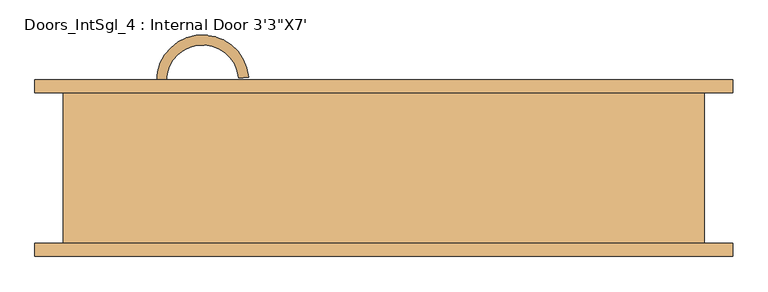
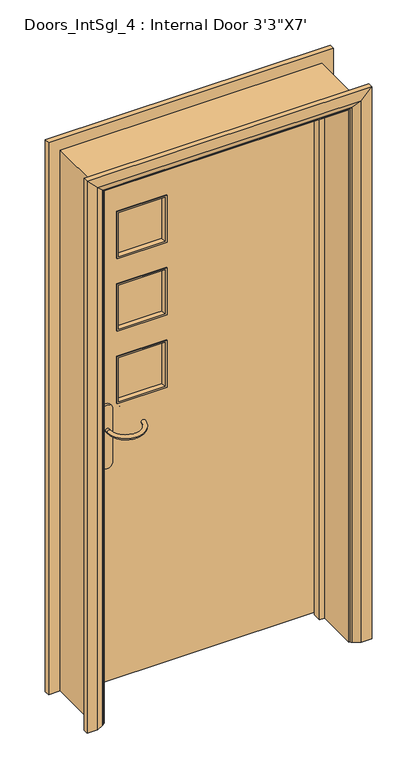
"""IFC4 building model written with IfcOpenShell, lengths in millimetres: door geometry."""

from ifc_helpers import new_model, si_unit, point, frame, frame_2d, origin, place, context, project, spatial, polyline, circle_curve, ellipse_curve, trimmed, segment, composite_curve, outline, extrude, faceted_brep, source, transform, mapped, element, save
from ifc_brep_helpers import plane_surface, cylinder_surface, revolved_surface, advanced_brep


def door_3dbecc4b(model_context):
    return source(origin(), model_context, "Body", "SolidModel", [
        advanced_brep(
        [(-345.5, 68.3, 1000.0), (-330.5, 68.3, 1000.0), (-330.5, 58.3, 1000.0), (-345.5, 58.3, 1000.0), (-205.5986682, 52.1917759, 1000.0), (-220.5415886, 53.4991121, 1000.0)],
        [
            (0, 1, circle_curve(frame((-338.0, 68.3, 1000.0), z_axis=(0.0, 1.0, 0.0), x_axis=(1.0, 0.0, 0.0)), 7.5)),
            (1, 0, circle_curve(frame((-338.0, 68.3, 1000.0), z_axis=(0.0, 1.0, 0.0), x_axis=(1.0, 0.0, 0.0)), 7.5)),
            (1, 2),
            (2, 3, circle_curve(frame((-338.0, 58.3, 1000.0), z_axis=(0.0, 1.0, 0.0), x_axis=(1.0, 0.0, 0.0)), 7.5)),
            (3, 0),
            (3, 2, circle_curve(frame((-338.0, 58.3, 1000.0), z_axis=(0.0, 1.0, 0.0), x_axis=(1.0, 0.0, 0.0)), 7.5)),
            (4, 5, circle_curve(frame((-213.0701284, 52.845444, 1000.0), z_axis=(0.08715574274766678, 0.9961946980917448, 0.0), x_axis=(-0.9961946980917448, 0.08715574274766678, 0.0)), 7.5)),
            (5, 4, circle_curve(frame((-213.0701284, 52.845444, 1000.0), z_axis=(0.08715574274766678, 0.9961946980917448, 0.0), x_axis=(-0.9961946980917448, 0.08715574274766678, 0.0)), 7.5)),
            (4, 3, circle_curve(frame((-275.4159887, 58.3, 1000.0), z_axis=(0.0, 0.0, -1.0), x_axis=(-1.0, 0.0, 0.0)), 70.0840113)),
            (2, 5, circle_curve(frame((-275.4159887, 58.3, 1000.0), z_axis=(0.0, 0.0, 1.0), x_axis=(-1.0, 0.0, 0.0)), 55.0840113)),
        ],
        [
            plane_surface(frame((-338.0, 68.3, 1000.0), z_axis=(0.0, 1.0, 0.0), x_axis=(0.0, 0.0, 1.0))),
            cylinder_surface(frame((-338.0, 68.3, 1000.0), z_axis=(0.0, 1.0, 0.0), x_axis=(1.0, 0.0, 0.0)), 7.5),
            plane_surface(frame((-213.0701284, 52.845444, 1000.0), z_axis=(0.08715574274766678, 0.9961946980917448, 0.0), x_axis=(0.0, 0.0, 1.0))),
            revolved_surface(trimmed(ellipse_curve(frame((-338.0, 58.3, 1000.0), z_axis=(0.0, -1.0, 0.0), x_axis=(1.0, 0.0, 0.0)), 7.5, 7.5), [point((-345.5, 58.3, 1000.0))], [point((-330.5, 58.3, 1000.0))], True, "CARTESIAN"), (-275.4159887, 58.3, 1000.0), (0.0, 0.0, -1.0)),
            revolved_surface(trimmed(ellipse_curve(frame((-338.0, 58.3, 1000.0), z_axis=(0.0, -1.0, 0.0), x_axis=(1.0, 0.0, 0.0)), 7.5, 7.5), [point((-330.5, 58.3, 1000.0))], [point((-345.5, 58.3, 1000.0))], True, "CARTESIAN"), (-275.4159887, 58.3, 1000.0), (0.0, 0.0, -1.0)),
        ],
        [
            (0, [[1, 2]]),
            (1, [[3, 4, 5, -2]]),
            (1, [[-5, 6, -3, -1]]),
            (2, [[7, 8]]),
            (3, [[-7, 9, -4, 10]]),
            (4, [[-8, -10, -6, -9]]),
        ],
    ),
        extrude(outline(composite_curve([segment(trimmed(circle_curve(frame_2d((870.0, -338.0)), 20.0), [point((870.0, -358.0))], [point((870.0, -318.0))], False, "CARTESIAN"), True, "CONTINUOUS"), segment(polyline([(870.0, -318.0), (1080.0, -318.0)]), True, "CONTINUOUS"), segment(trimmed(circle_curve(frame_2d((1080.0, -338.0)), 20.0), [point((1080.0, -318.0))], [point((1080.0, -358.0))], False, "CARTESIAN"), True, "CONTINUOUS"), segment(polyline([(1080.0, -358.0), (870.0, -358.0)]), True, "CONTINUOUS")], self_intersect=False)), frame((0.0, 68.3, 0.0), z_axis=(0.0, 1.0, 0.0), x_axis=(0.0, 0.0, 1.0)), (0.0, 0.0, 1.0), 8.0),
        advanced_brep(
        [(-345.5, 122.3, 1000.0), (-330.5, 122.3, 1000.0), (-345.5, 132.3, 1000.0), (-330.5, 132.3, 1000.0), (-205.5986682, 138.4082241, 1000.0), (-220.5415886, 137.1008879, 1000.0)],
        [
            (0, 1, circle_curve(frame((-338.0, 122.3, 1000.0), z_axis=(0.0, -1.0, 0.0), x_axis=(1.0, 0.0, 0.0)), 7.5)),
            (1, 0, circle_curve(frame((-338.0, 122.3, 1000.0), z_axis=(0.0, -1.0, 0.0), x_axis=(1.0, 0.0, 0.0)), 7.5)),
            (0, 2),
            (2, 3, circle_curve(frame((-338.0, 132.3, 1000.0), z_axis=(0.0, -1.0, 0.0), x_axis=(1.0, 0.0, 0.0)), 7.5)),
            (3, 1),
            (3, 2, circle_curve(frame((-338.0, 132.3, 1000.0), z_axis=(0.0, -1.0, 0.0), x_axis=(1.0, 0.0, 0.0)), 7.5)),
            (4, 5, circle_curve(frame((-213.0701284, 137.754556, 1000.0), z_axis=(0.08715574274766356, -0.9961946980917451, 0.0), x_axis=(-0.9961946980917451, -0.08715574274766356, 0.0)), 7.5)),
            (5, 4, circle_curve(frame((-213.0701284, 137.754556, 1000.0), z_axis=(0.08715574274766356, -0.9961946980917451, 0.0), x_axis=(-0.9961946980917451, -0.08715574274766356, 0.0)), 7.5)),
            (5, 3, circle_curve(frame((-275.4159887, 132.3, 1000.0), z_axis=(0.0, 0.0, 1.0), x_axis=(-1.0, 0.0, 0.0)), 55.0840113)),
            (2, 4, circle_curve(frame((-275.4159887, 132.3, 1000.0), z_axis=(0.0, 0.0, -1.0), x_axis=(-1.0, 0.0, 0.0)), 70.0840113)),
        ],
        [
            plane_surface(frame((-338.0, 122.3, 1000.0), z_axis=(0.0, -1.0, 0.0), x_axis=(0.0, 0.0, 1.0))),
            cylinder_surface(frame((-338.0, 122.3, 1000.0), z_axis=(0.0, -1.0, 0.0), x_axis=(1.0, 0.0, 0.0)), 7.5),
            plane_surface(frame((-213.0701284, 137.754556, 1000.0), z_axis=(0.08715574274766356, -0.9961946980917451, 0.0), x_axis=(0.0, 0.0, 1.0))),
            revolved_surface(trimmed(ellipse_curve(frame((-338.0, 132.3, 1000.0), z_axis=(0.0, -1.0, 0.0), x_axis=(1.0, 0.0, 0.0)), 7.5, 7.5), [point((-345.5, 132.3, 1000.0))], [point((-330.5, 132.3, 1000.0))], True, "CARTESIAN"), (-275.4159887, 132.3, 1000.0), (0.0, 0.0, -1.0)),
            revolved_surface(trimmed(ellipse_curve(frame((-338.0, 132.3, 1000.0), z_axis=(0.0, -1.0, 0.0), x_axis=(1.0, 0.0, 0.0)), 7.5, 7.5), [point((-330.5, 132.3, 1000.0))], [point((-345.5, 132.3, 1000.0))], True, "CARTESIAN"), (-275.4159887, 132.3, 1000.0), (0.0, 0.0, -1.0)),
        ],
        [
            (0, [[1, 2]]),
            (1, [[-1, 3, 4, 5]]),
            (1, [[-2, -5, 6, -3]]),
            (2, [[7, 8]]),
            (3, [[9, -4, 10, -8]]),
            (4, [[-10, -6, -9, -7]]),
        ],
    ),
        extrude(outline(composite_curve([segment(trimmed(circle_curve(frame_2d((870.0, -338.0)), 20.0), [point((870.0, -358.0))], [point((870.0, -318.0))], False, "CARTESIAN"), True, "CONTINUOUS"), segment(polyline([(870.0, -318.0), (1080.0, -318.0)]), True, "CONTINUOUS"), segment(trimmed(circle_curve(frame_2d((1080.0, -338.0)), 20.0), [point((1080.0, -318.0))], [point((1080.0, -358.0))], False, "CARTESIAN"), True, "CONTINUOUS"), segment(polyline([(1080.0, -358.0), (870.0, -358.0)]), True, "CONTINUOUS")], self_intersect=False)), frame((0.0, 114.3, 0.0), z_axis=(0.0, 1.0, 0.0), x_axis=(0.0, 0.0, 1.0)), (0.0, 0.0, 1.0), 8.0),
        extrude(outline(polyline([(2091.6, -453.3), (8.0, -453.3), (8.0, 453.3), (2091.6, 453.3), (2091.6, -453.3)]), holes=[polyline([(1841.6, -113.3), (1656.6, -113.3), (1656.6, -298.3), (1841.6, -298.3), (1841.6, -113.3)]), polyline([(1086.6, -298.3), (1271.6, -298.3), (1271.6, -113.3), (1086.6, -113.3), (1086.6, -298.3)]), polyline([(1556.6, -113.3), (1371.6, -113.3), (1371.6, -298.3), (1556.6, -298.3), (1556.6, -113.3)])]), frame((0.0, 76.3, 0.0), z_axis=(0.0, 1.0, 0.0), x_axis=(0.0, 0.0, 1.0)), (0.0, 0.0, 1.0), 38.0),
        faceted_brep([(-455.3, 114.3, 0.0), (-455.3, -114.3, 0.0), (-487.3, -114.3, 0.0), (-487.3, 114.3, 0.0), (-455.3, 114.3, 2093.6), (-455.3, -114.3, 2093.6), (-487.3, -114.3, 2125.6), (-487.3, 114.3, 2125.6), (455.3, 114.3, 0.0), (487.3, 114.3, 0.0), (487.3, -114.3, 0.0), (455.3, -114.3, 0.0), (455.3, 114.3, 2093.6), (487.3, 114.3, 2125.6), (487.3, -114.3, 2125.6), (455.3, -114.3, 2093.6)], [[[0, 1, 2, 3]], [[1, 0, 4, 5]], [[2, 1, 5, 6]], [[3, 2, 6, 7]], [[0, 3, 7, 4]], [[8, 9, 10, 11]], [[12, 13, 9, 8]], [[13, 14, 10, 9]], [[14, 15, 11, 10]], [[15, 12, 8, 11]], [[5, 4, 12, 15]], [[6, 5, 15, 14]], [[7, 6, 14, 13]], [[4, 7, 13, 12]]]),
        advanced_brep(
        [(-530.3, -134.3, 0.0), (-530.3, -114.3, 0.0), (-460.3, -114.3, 0.0), (-464.3, -120.3, 0.0), (-490.3, -134.3, 0.0), (-530.3, -134.3, 2168.6), (-530.3, -114.3, 2168.6), (-460.3, -114.3, 2098.6), (-464.3, -120.3, 2102.6), (-490.3, -134.3, 2128.6), (530.3, -134.3, 0.0), (490.3, -134.3, 0.0), (464.3, -120.3, 0.0), (460.3, -114.3, 0.0), (530.3, -114.3, 0.0), (530.3, -134.3, 2168.6), (490.3, -134.3, 2128.6), (464.3, -120.3, 2102.6), (460.3, -114.3, 2098.6), (530.3, -114.3, 2168.6)],
        [
            (0, 1),
            (1, 2),
            (2, 3, circle_curve(frame((-468.3, -113.3, 0.0), z_axis=(0.0, 0.0, -1.0), x_axis=(-1.0, 0.0, 0.0)), 8.0622577)),
            (3, 4),
            (4, 0),
            (0, 5),
            (5, 6),
            (6, 1),
            (6, 7),
            (7, 2),
            (7, 8, ellipse_curve(frame((-468.3, -113.3, 2106.6), z_axis=(-0.7071067811865475, 0.0, -0.7071067811865475), x_axis=(0.7071067811865474, 0.0, -0.7071067811865476)), 11.4017543, 8.0622577)),
            (8, 3),
            (8, 9),
            (9, 4),
            (9, 5),
            (10, 11),
            (11, 12),
            (12, 13, circle_curve(frame((468.3, -113.3, 0.0), z_axis=(0.0, 0.0, -1.0), x_axis=(1.0, 0.0, 0.0)), 8.0622577)),
            (13, 14),
            (14, 10),
            (15, 16),
            (16, 11),
            (10, 15),
            (16, 17),
            (17, 12),
            (17, 18, ellipse_curve(frame((468.3, -113.3, 2106.6), z_axis=(0.7071067811865475, 0.0, -0.7071067811865475), x_axis=(0.7071067811865474, 0.0, 0.7071067811865476)), 11.4017543, 8.0622577)),
            (18, 13),
            (18, 19),
            (19, 14),
            (19, 15),
            (5, 15),
            (19, 6),
            (18, 7),
            (17, 8),
            (16, 9),
        ],
        [
            plane_surface(frame((-460.3, -187.1010989, 0.0), z_axis=(0.0, 0.0, -1.0), x_axis=(1.0, 0.0, 0.0))),
            plane_surface(frame((-530.3, -134.3, 0.0), z_axis=(-1.0, 0.0, 0.0), x_axis=(0.0, 0.0, 1.0))),
            plane_surface(frame((-530.3, -114.3, 0.0), z_axis=(0.0, 1.0, 0.0), x_axis=(0.0, 0.0, 1.0))),
            cylinder_surface(frame((-468.3, -113.3, 0.0), z_axis=(0.0, 0.0, -1.0), x_axis=(-1.0, 0.0, 0.0)), 8.0622577),
            plane_surface(frame((-464.3, -120.3, 0.0), z_axis=(0.4740998230350183, -0.8804710999221749, 0.0), x_axis=(0.0, 0.0, 1.0))),
            plane_surface(frame((-490.3, -134.3, 0.0), z_axis=(0.0, -1.0, 0.0), x_axis=(0.0, 0.0, 1.0))),
            plane_surface(frame((460.3, -187.1010989, 0.0), z_axis=(0.0, 0.0, -1.0), x_axis=(-1.0, 0.0, 0.0))),
            plane_surface(frame((490.3, -134.3, 2128.6), z_axis=(0.0, -1.0, 0.0), x_axis=(0.0, 0.0, -1.0))),
            plane_surface(frame((464.3, -120.3, 2102.6), z_axis=(-0.4740998230350183, -0.8804710999221749, 0.0), x_axis=(0.0, 0.0, -1.0))),
            cylinder_surface(frame((468.3, -113.3, 2098.6), z_axis=(0.0, 0.0, 1.0), x_axis=(1.0, 0.0, 0.0)), 8.0622577),
            plane_surface(frame((530.3, -114.3, 2168.6), z_axis=(0.0, 1.0, 0.0), x_axis=(0.0, 0.0, -1.0))),
            plane_surface(frame((530.3, -134.3, 2168.6), z_axis=(1.0, 0.0, 0.0), x_axis=(0.0, 0.0, -1.0))),
            plane_surface(frame((-530.3, -134.3, 2168.6), z_axis=(0.0, 0.0, 1.0), x_axis=(1.0, 0.0, 0.0))),
            plane_surface(frame((-530.3, -114.3, 2168.6), z_axis=(0.0, 1.0, 0.0), x_axis=(1.0, 0.0, 0.0))),
            cylinder_surface(frame((-460.3, -113.3, 2106.6), z_axis=(-1.0, 0.0, 0.0), x_axis=(0.0, 0.0, 1.0)), 8.0622577),
            plane_surface(frame((-464.3, -120.3, 2102.6), z_axis=(0.0, -0.8804710999221749, -0.4740998230350183), x_axis=(1.0, 0.0, 0.0))),
            plane_surface(frame((-490.3, -134.3, 2128.6), z_axis=(0.0, -1.0, 0.0), x_axis=(1.0, 0.0, 0.0))),
        ],
        [
            (0, [[1, 2, 3, 4, 5]]),
            (1, [[-1, 6, 7, 8]]),
            (2, [[-2, -8, 9, 10]]),
            (3, [[-3, -10, 11, 12]]),
            (4, [[-4, -12, 13, 14]]),
            (5, [[-5, -14, 15, -6]]),
            (6, [[16, 17, 18, 19, 20]]),
            (7, [[21, 22, -16, 23]]),
            (8, [[24, 25, -17, -22]]),
            (9, [[26, 27, -18, -25]]),
            (10, [[28, 29, -19, -27]]),
            (11, [[30, -23, -20, -29]]),
            (12, [[-7, 31, -30, 32]]),
            (13, [[-9, -32, -28, 33]]),
            (14, [[-11, -33, -26, 34]]),
            (15, [[-13, -34, -24, 35]]),
            (16, [[-15, -35, -21, -31]]),
        ],
    ),
        extrude(outline(polyline([(0.0, -455.3), (0.0, -436.3), (2074.6, -436.3), (2074.6, 436.3), (0.0, 436.3), (0.0, 455.3), (2093.6, 455.3), (2093.6, -455.3), (0.0, -455.3)])), frame((0.0, 42.3, 0.0), z_axis=(0.0, 1.0, 0.0), x_axis=(0.0, 0.0, 1.0)), (0.0, 0.0, 1.0), 32.0),
        advanced_brep(
        [(530.3, 134.3, 0.0), (530.3, 114.3, 0.0), (460.3, 114.3, 0.0), (464.3, 120.3, 0.0), (490.3, 134.3, 0.0), (530.3, 134.3, 2168.6), (530.3, 114.3, 2168.6), (-530.3, 114.3, 2168.6), (-530.3, 114.3, 0.0), (-460.3, 114.3, 0.0), (-460.3, 114.3, 2098.6), (460.3, 114.3, 2098.6), (464.3, 120.3, 2102.6), (490.3, 134.3, 2128.6), (-490.3, 134.3, 2128.6), (-490.3, 134.3, 0.0), (-530.3, 134.3, 0.0), (-530.3, 134.3, 2168.6), (-464.3, 120.3, 0.0), (-464.3, 120.3, 2102.6)],
        [
            (0, 1),
            (1, 2),
            (2, 3, circle_curve(frame((468.3, 113.3, 0.0), z_axis=(0.0, 0.0, -1.0), x_axis=(1.0, 0.0, 0.0)), 8.0622577)),
            (3, 4),
            (4, 0),
            (0, 5),
            (5, 6),
            (6, 1),
            (6, 7),
            (7, 8),
            (8, 9),
            (9, 10),
            (10, 11),
            (11, 2),
            (11, 12, ellipse_curve(frame((468.3, 113.3, 2106.6), z_axis=(0.7071067811865475, 0.0, -0.7071067811865475), x_axis=(-0.7071067811865474, 0.0, -0.7071067811865476)), 11.4017543, 8.0622577)),
            (12, 3),
            (12, 13),
            (13, 4),
            (13, 14),
            (14, 15),
            (15, 16),
            (16, 17),
            (17, 5),
            (7, 17),
            (16, 8),
            (15, 18),
            (18, 9, circle_curve(frame((-468.3, 113.3, 0.0), z_axis=(0.0, 0.0, -1.0), x_axis=(-1.0, 0.0, 0.0)), 8.0622577)),
            (19, 10, ellipse_curve(frame((-468.3, 113.3, 2106.6), z_axis=(-0.7071067811865475, 0.0, -0.7071067811865475), x_axis=(-0.7071067811865474, 0.0, 0.7071067811865476)), 11.4017543, 8.0622577)),
            (18, 19),
            (14, 19),
            (19, 12),
        ],
        [
            plane_surface(frame((460.3, 114.3, 0.0), z_axis=(0.0, 0.0, -1.0), x_axis=(0.0, -1.0, 0.0))),
            plane_surface(frame((530.3, 134.3, 0.0), z_axis=(1.0, 0.0, 0.0), x_axis=(0.0, 0.0, 1.0))),
            plane_surface(frame((530.3, 114.3, 0.0), z_axis=(0.0, -1.0, 0.0), x_axis=(0.0, 0.0, 1.0))),
            cylinder_surface(frame((468.3, 113.3, 0.0), z_axis=(0.0, 0.0, -1.0), x_axis=(1.0, 0.0, 0.0)), 8.0622577),
            plane_surface(frame((464.3, 120.3, 0.0), z_axis=(-0.4740998230350126, 0.8804710999221779, 0.0), x_axis=(0.0, 0.0, 1.0))),
            plane_surface(frame((490.3, 134.3, 0.0), z_axis=(0.0, 1.0, 0.0), x_axis=(0.0, 0.0, 1.0))),
            plane_surface(frame((-530.3, 134.3, 2168.6), z_axis=(-1.0, 0.0, 0.0), x_axis=(0.0, 0.0, -1.0))),
            plane_surface(frame((-460.3, 114.3, 0.0), z_axis=(0.0, 0.0, -1.0), x_axis=(0.0, -1.0, 0.0))),
            cylinder_surface(frame((-468.3, 113.3, 2098.6), z_axis=(0.0, 0.0, 1.0), x_axis=(-1.0, 0.0, 0.0)), 8.0622577),
            plane_surface(frame((-464.3, 120.3, 2102.6), z_axis=(0.4740998230350183, 0.8804710999221749, 0.0), x_axis=(0.0, 0.0, -1.0))),
            plane_surface(frame((530.3, 134.3, 2168.6), z_axis=(0.0, 0.0, 1.0), x_axis=(-1.0, 0.0, 0.0))),
            cylinder_surface(frame((460.3, 113.3, 2106.6), z_axis=(1.0, 0.0, 0.0), x_axis=(0.0, 0.0, 1.0)), 8.0622577),
            plane_surface(frame((464.3, 120.3, 2102.6), z_axis=(0.0, 0.8804710999221763, -0.4740998230350154), x_axis=(-1.0, 0.0, 0.0))),
        ],
        [
            (0, [[1, 2, 3, 4, 5]]),
            (1, [[-1, 6, 7, 8]]),
            (2, [[-2, -8, 9, 10, 11, 12, 13, 14]]),
            (3, [[-3, -14, 15, 16]]),
            (4, [[-4, -16, 17, 18]]),
            (5, [[-5, -18, 19, 20, 21, 22, 23, -6]]),
            (6, [[24, -22, 25, -10]]),
            (7, [[-21, 26, 27, -11, -25]]),
            (8, [[28, -12, -27, 29]]),
            (9, [[30, -29, -26, -20]]),
            (10, [[-7, -23, -24, -9]]),
            (11, [[-15, -13, -28, 31]]),
            (12, [[-17, -31, -30, -19]]),
        ],
    ),
        faceted_brep([(-113.3, 117.3, 1841.6), (-113.3, 104.3, 1841.6), (-113.3, 104.3, 1656.6), (-113.3, 117.3, 1656.6), (-125.3, 104.3, 1829.6), (-119.3, 117.3, 1835.6), (-119.3, 117.3, 1662.6), (-125.3, 104.3, 1668.6), (-298.3, 104.3, 1656.6), (-298.3, 117.3, 1656.6), (-292.3, 117.3, 1662.6), (-286.3, 104.3, 1668.6), (-298.3, 104.3, 1841.6), (-298.3, 117.3, 1841.6), (-292.3, 117.3, 1835.6), (-286.3, 104.3, 1829.6)], [[[0, 1, 2, 3]], [[4, 5, 6, 7]], [[3, 2, 8, 9]], [[7, 6, 10, 11]], [[9, 8, 12, 13]], [[11, 10, 14, 15]], [[1, 12, 8, 2], [7, 11, 15, 4]], [[13, 12, 1, 0]], [[3, 9, 13, 0], [5, 14, 10, 6]], [[15, 14, 5, 4]]]),
        faceted_brep([(-119.3, 73.3, 1835.6), (-125.3, 86.3, 1829.6), (-125.3, 86.3, 1668.6), (-119.3, 73.3, 1662.6), (-113.3, 86.3, 1841.6), (-113.3, 73.3, 1841.6), (-113.3, 73.3, 1656.6), (-113.3, 86.3, 1656.6), (-286.3, 86.3, 1668.6), (-292.3, 73.3, 1662.6), (-298.3, 73.3, 1656.6), (-298.3, 86.3, 1656.6), (-286.3, 86.3, 1829.6), (-292.3, 73.3, 1835.6), (-298.3, 73.3, 1841.6), (-298.3, 86.3, 1841.6)], [[[0, 1, 2, 3]], [[4, 5, 6, 7]], [[3, 2, 8, 9]], [[7, 6, 10, 11]], [[9, 8, 12, 13]], [[11, 10, 14, 15]], [[13, 12, 1, 0]], [[5, 14, 10, 6], [3, 9, 13, 0]], [[15, 14, 5, 4]], [[7, 11, 15, 4], [1, 12, 8, 2]]]),
        extrude(outline(polyline([(-298.3, 104.3), (-113.3, 104.3), (-113.3, 86.3), (-298.3, 86.3), (-298.3, 104.3)])), frame((0.0, 0.0, 1656.6), z_axis=(0.0, 0.0, 1.0), x_axis=(1.0, 0.0, 0.0)), (0.0, 0.0, 1.0), 185.0),
        extrude(outline(polyline([(-298.3, 104.3), (-113.3, 104.3), (-113.3, 86.3), (-298.3, 86.3), (-298.3, 104.3)])), frame((0.0, 0.0, 1086.6), z_axis=(0.0, 0.0, 1.0), x_axis=(1.0, 0.0, 0.0)), (0.0, 0.0, 1.0), 185.0),
        extrude(outline(polyline([(-298.3, 104.3), (-113.3, 104.3), (-113.3, 86.3), (-298.3, 86.3), (-298.3, 104.3)])), frame((0.0, 0.0, 1371.6), z_axis=(0.0, 0.0, 1.0), x_axis=(1.0, 0.0, 0.0)), (0.0, 0.0, 1.0), 185.0),
        faceted_brep([(-298.3, 117.3, 1371.6), (-298.3, 104.3, 1371.6), (-298.3, 104.3, 1556.6), (-298.3, 117.3, 1556.6), (-286.3, 104.3, 1383.6), (-292.3, 117.3, 1377.6), (-292.3, 117.3, 1550.6), (-286.3, 104.3, 1544.6), (-113.3, 104.3, 1556.6), (-113.3, 117.3, 1556.6), (-119.3, 117.3, 1550.6), (-125.3, 104.3, 1544.6), (-113.3, 104.3, 1371.6), (-113.3, 117.3, 1371.6), (-119.3, 117.3, 1377.6), (-125.3, 104.3, 1383.6)], [[[0, 1, 2, 3]], [[4, 5, 6, 7]], [[3, 2, 8, 9]], [[7, 6, 10, 11]], [[9, 8, 12, 13]], [[11, 10, 14, 15]], [[1, 12, 8, 2], [7, 11, 15, 4]], [[13, 12, 1, 0]], [[3, 9, 13, 0], [5, 14, 10, 6]], [[15, 14, 5, 4]]]),
        faceted_brep([(-298.3, 117.3, 1086.6), (-298.3, 104.3, 1086.6), (-298.3, 104.3, 1271.6), (-298.3, 117.3, 1271.6), (-286.3, 104.3, 1098.6), (-292.3, 117.3, 1092.6), (-292.3, 117.3, 1265.6), (-286.3, 104.3, 1259.6), (-113.3, 104.3, 1271.6), (-113.3, 117.3, 1271.6), (-119.3, 117.3, 1265.6), (-125.3, 104.3, 1259.6), (-113.3, 104.3, 1086.6), (-113.3, 117.3, 1086.6), (-119.3, 117.3, 1092.6), (-125.3, 104.3, 1098.6)], [[[0, 1, 2, 3]], [[4, 5, 6, 7]], [[3, 2, 8, 9]], [[7, 6, 10, 11]], [[9, 8, 12, 13]], [[11, 10, 14, 15]], [[1, 12, 8, 2], [7, 11, 15, 4]], [[13, 12, 1, 0]], [[3, 9, 13, 0], [5, 14, 10, 6]], [[15, 14, 5, 4]]]),
        faceted_brep([(-113.3, 73.3, 1371.6), (-113.3, 86.3, 1371.6), (-113.3, 86.3, 1556.6), (-113.3, 73.3, 1556.6), (-125.3, 86.3, 1383.6), (-119.3, 73.3, 1377.6), (-119.3, 73.3, 1550.6), (-125.3, 86.3, 1544.6), (-298.3, 86.3, 1556.6), (-298.3, 73.3, 1556.6), (-292.3, 73.3, 1550.6), (-286.3, 86.3, 1544.6), (-298.3, 86.3, 1371.6), (-298.3, 73.3, 1371.6), (-292.3, 73.3, 1377.6), (-286.3, 86.3, 1383.6)], [[[0, 1, 2, 3]], [[4, 5, 6, 7]], [[3, 2, 8, 9]], [[7, 6, 10, 11]], [[9, 8, 12, 13]], [[11, 10, 14, 15]], [[1, 12, 8, 2], [7, 11, 15, 4]], [[13, 12, 1, 0]], [[3, 9, 13, 0], [5, 14, 10, 6]], [[15, 14, 5, 4]]]),
        faceted_brep([(-113.3, 73.3, 1086.6), (-113.3, 86.3, 1086.6), (-113.3, 86.3, 1271.6), (-113.3, 73.3, 1271.6), (-125.3, 86.3, 1098.6), (-119.3, 73.3, 1092.6), (-119.3, 73.3, 1265.6), (-125.3, 86.3, 1259.6), (-298.3, 86.3, 1271.6), (-298.3, 73.3, 1271.6), (-292.3, 73.3, 1265.6), (-286.3, 86.3, 1259.6), (-298.3, 86.3, 1086.6), (-298.3, 73.3, 1086.6), (-292.3, 73.3, 1092.6), (-286.3, 86.3, 1098.6)], [[[0, 1, 2, 3]], [[4, 5, 6, 7]], [[3, 2, 8, 9]], [[7, 6, 10, 11]], [[9, 8, 12, 13]], [[11, 10, 14, 15]], [[1, 12, 8, 2], [7, 11, 15, 4]], [[13, 12, 1, 0]], [[3, 9, 13, 0], [5, 14, 10, 6]], [[15, 14, 5, 4]]]),
    ])


if __name__ == "__main__":
    model = new_model("IFC4")
    model_context = context("Model", 3, world=origin())
    ifc_project = project(units=[si_unit("LENGTHUNIT", "METRE", prefix="MILLI")], contexts=[model_context])
    site = spatial("IfcSite", under=ifc_project)
    building = spatial("IfcBuilding", under=site)
    placement = place(None, origin())
    door_shape = door_3dbecc4b(model_context)
    element("IfcDoor", 1, ObjectType="Doors_IntSgl_4 : Internal Door 3'3\"X7'", at=placement, inside=building, context=model_context, shape_type="MappedRepresentation", body=[
        mapped(door_shape, transform((0.0, 0.0, 0.0), x_axis=(1.0, 0.0, 0.0), y_axis=(0.0, 1.0, 0.0), z_axis=(0.0, 0.0, 1.0))),
    ])
    save(model, "model.ifc")

# Revit data of these elements
# Type "Doors_IntSgl_4 : Internal Door 3'3\"X7'"
#   Type Mark = "13"
#   Type Comments = "Internal Single"
#   Operation = "SingleSwingRight"
#   Construction Type Id = "SGL"
#   Manufacturer = "Revit"
#   Keynote = "L20"
#   Description = "Internal Single Door"
#   Analytic Construction = "Large single-glazed windows"
#   Visual Light Transmittance = 0.9
#   VisionPanel Width = 0' - 7.28346"
#   VisionPanel Depth = 0' - 7.28346"
#   UnderCut = 0' - 0.31496"
#   Tolerance = 0' - 0.07874"
#   Thickness = 0' - 1.49606"
#   Structural Tolerance = 0' - 0.31496"
#   StopDepth = 0' - 1.25984"
#   Stop Thickness = 0' - 0.74803"
#   Stile Shutting = 0' - 6.10236"
#   Stile Top Rail = 0' - 9.84252"
#   Stile Intermediate/Frieze = 0' - 3.93701"
#   Solar Heat Gain Coefficient = 0.86
#   Rough Width = 3' - 3"
#   Rough Height = 7' - 0"
#   Heat Transfer Coefficient (U) = 0.979472 BTU/(h·ft²·°F)
#   Handle Z Distance = 3' - 3.37008"
#   Handle X Distance = 0' - 2.95276"
#   Handle Length = 1' - 1.77953"
#   Frame Thickness = 0' - 1.25984"
#   Door Panel Width = 2' - 11.69291"
#   Door Panel Thickness = 0' - 1.49606"
#   Door Panel Offset = 0' - 0"
#   Height = 7' - 0"
#   Width = 3' - 3"
#   Door Panel Height = 6' - 10.0315"
#   Architrave Setback = 0' - 0.19685"
#   Vis - Ironmongery = yes
#   Define Thermal Properties by = 1
#   Material Ironmongery = Door - Handle
#   Material Glass = Door - Glazing
#   Material Frame = Door - Frame/Mullion
#   Material Door = Door - Panel
#   Material Beading = Door - Panel
#   Material Architrave = Door - Architrave
#   Handle Style = element 386699
#   Function = (empty or 0)
#   Wall Closure = (empty or 0)
# Element 1 (IfcDoor, "Doors_IntSgl_4 : Internal Door 3'3\"X7'")
#   Materials on its faces: "Door - Panel", "Door - Architrave", "Door - Handle", "Door - Frame/Mullion", "Door - Glazing"
# Materials
#   "Door - Handle": colour RGB 247 247 247, transparency 0
#   "Door - Glazing": colour RGB 0 0 255, transparency 0.75
#   "Door - Frame/Mullion": class "Wood", colour RGB 212 179 113, transparency 0
#   "Door - Panel": class "Wood", colour RGB 210 159 95, transparency 0, Cost = 0
#   "Door - Architrave": class "Wood", colour RGB 212 179 113, transparency 0
